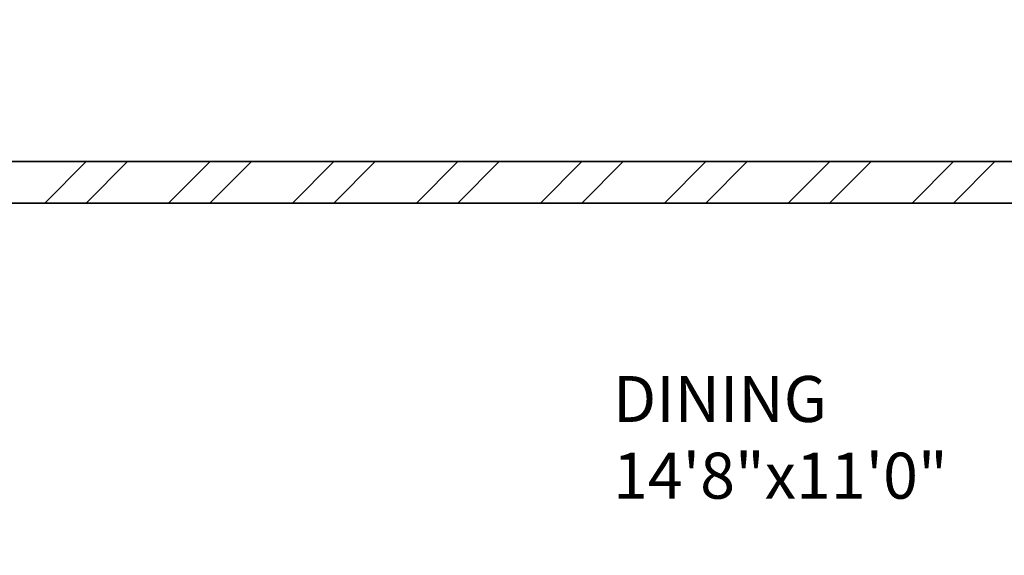
# Model space of a CAD drawing. Units: inches. Extents: x 1885 to 2748, y 783 to 2421.
# Tile 27 of 117: x 2338 to 2445, y 1292 to 1350. Entities that reach past the tile are written whole.
import ezdxf

# ---------------------------------------------------------------- set-up
doc = ezdxf.new("R2010")
doc.units = ezdxf.units.IN
doc.layers.add('A-AREA-IDEN', color=7, linetype='Continuous', lineweight=18)
doc.layers.add('A-WALL', color=7, linetype='Continuous', lineweight=35)
doc.layers.add('A-WALL-PATT', color=85, linetype='Continuous', lineweight=13, true_color=0x58ba48)
doc.styles.get("Standard").update_dxf_attribs({"font": 'arial.ttf'})

msp = doc.modelspace()

# ---------------------------------------------------------------- hatches: boundary and pattern name
at = {"layer": 'A-WALL-PATT'}
h = msp.add_hatch(dxfattribs=at)
h.set_pattern_fill('ANSI32', color=256)
h.paths.add_polyline_path([(2007.77, 2318.01), (1980.77, 2318.01), (1980.77, 2281.22), (1985.27, 2281.22), (1985.27, 2313.51), (2007.77, 2313.51), (2007.77, 2315.76)])
h.paths.add_polyline_path([(2094.32, 2318.01), (2067.77, 2318.01), (2067.77, 2313.51), (2094.32, 2313.51), (2094.32, 2315.76)])
h.paths.add_polyline_path([(2131.37, 2315.76), (2131.37, 2318.01), (2131.19, 2318.01), (2112.61, 2318.01), (2112.61, 2313.51), (2117.27, 2313.51), (2117.27, 2255.2), (2121.77, 2255.2), (2121.77, 2313.51), (2131.37, 2313.51)])
h.paths.add_polyline_path([(2190.51, 2318.01), (2155.37, 2318.01), (2155.37, 2313.51), (2169.77, 2313.51), (2169.77, 2229.51), (2121.77, 2229.51), (2121.77, 2233.45), (2119.52, 2233.45), (2117.27, 2233.45), (2117.27, 2201.1), (2121.77, 2201.1), (2121.77, 2225.01), (2169.77, 2225.01), (2169.77, 2165.01), (2306.27, 2165.01), (2306.27, 2066.01), (2310.77, 2066.01), (2344.27, 2066.01), (2486.27, 2066.01), (2486.27, 1886.01), (2483.02, 1886.01), (2483.02, 1881.51), (2486.27, 1881.51), (2486.27, 1880.68), (2490.77, 1880.68), (2490.77, 2070.51), (2344.27, 2070.51), (2310.77, 2070.51), (2310.77, 2165.01), (2310.77, 2173.64), (2308.52, 2173.64), (2306.27, 2173.64), (2306.27, 2169.51), (2174.27, 2169.51), (2174.27, 2313.51), (2190.51, 2313.51), (2190.51, 2315.76)])
h.paths.add_polyline_path([(1985.27, 2221.22), (1980.77, 2221.22), (1980.77, 2165.01), (1992.77, 2165.01), (1992.77, 2141.93), (1997.27, 2141.93), (1997.27, 2165.01), (2117.27, 2165.01), (2117.27, 2163.13), (2121.77, 2163.13), (2121.77, 2172.73), (2119.52, 2172.73), (2117.27, 2172.73), (2117.27, 2169.51), (1985.27, 2169.51)])
h.paths.add_polyline_path([(1997.27, 2105.93), (1992.77, 2105.93), (1992.77, 2070.51), (2016.77, 2070.51), (2016.77, 2059.12), (2019.02, 2059.12), (2021.27, 2059.12), (2021.27, 2070.51), (2117.27, 2070.51), (2117.27, 2022.51), (2114.42, 2022.51), (2114.42, 2018.01), (2123.63, 2018.01), (2123.63, 2020.26), (2123.63, 2022.51), (2121.77, 2022.51), (2121.77, 2142.59), (2119.52, 2142.59), (2117.27, 2142.59), (2117.27, 2075.01), (1997.27, 2075.01)])
h.paths.add_polyline_path([(2092.03, 2020.26), (2092.03, 2022.51), (2021.27, 2022.51), (2021.27, 2035.12), (2016.77, 2035.12), (2016.77, 2018.01), (2016.77, 1978.78), (2021.27, 1978.78), (2021.27, 2018.01), (2092.03, 2018.01)])
h.paths.add_polyline_path([(2260.94, 2022.51), (2153.1, 2022.51), (2153.1, 2020.26), (2153.1, 2018.01), (2155.27, 2018.01), (2155.27, 1886.01), (2107.63, 1886.01), (2107.63, 1881.51), (2182.91, 1881.51), (2182.91, 1883.76), (2182.91, 1886.01), (2159.77, 1886.01), (2159.77, 2018.01), (2260.94, 2018.01), (2260.94, 2020.26)])
h.paths.add_polyline_path([(2047.63, 1883.76), (2047.63, 1886.01), (2021.27, 1886.01), (2021.27, 1918.78), (2019.02, 1918.78), (2016.77, 1918.78), (2016.77, 1881.51), (2047.63, 1881.51)])
h.paths.add_polyline_path([(2306.36, 1883.76), (2306.36, 1886.01), (2296.27, 1886.01), (2296.27, 1982.01), (2316.54, 1982.01), (2316.54, 1984.26), (2316.54, 1986.51), (2296.27, 1986.51), (2296.27, 2022.51), (2289.28, 2022.51), (2289.28, 2018.01), (2291.77, 2018.01), (2291.77, 1886.01), (2242.91, 1886.01), (2242.91, 1881.51), (2306.36, 1881.51)], flags=17)
h.paths.add_polyline_path([(1985.27, 1843.01), (2021.6, 1843.01), (2021.53, 1845.44), (2021.48, 1847.51), (1980.77, 1847.51), (1980.77, 1809.45), (1985.27, 1809.45)])
h.paths.add_polyline_path([(2131.48, 1845.26), (2131.48, 1847.51), (2081.53, 1847.51), (2081.53, 1843.01), (2117.27, 1843.01), (2117.27, 1784.15), (2119.52, 1784.15), (2121.77, 1784.15), (2121.77, 1843.01), (2131.48, 1843.01)])
h.paths.add_polyline_path([(2203.89, 1847.51), (2155.48, 1847.51), (2155.48, 1843.01), (2169.77, 1843.01), (2169.77, 1759.01), (2121.77, 1759.01), (2121.77, 1761.46), (2117.27, 1761.46), (2117.27, 1730.43), (2121.77, 1730.43), (2121.77, 1754.51), (2177.42, 1754.51), (2177.42, 1756.76), (2177.42, 1759.01), (2174.27, 1759.01), (2174.27, 1843.01), (2203.89, 1843.01)])
h.paths.add_polyline_path([(2335.55, 1845.26), (2335.55, 1847.51), (2239.89, 1847.51), (2239.89, 1843.01), (2306.27, 1843.01), (2306.27, 1759.01), (2199.49, 1759.01), (2199.49, 1754.51), (2310.77, 1754.51), (2310.77, 1843.01), (2335.55, 1843.01)])
h.paths.add_polyline_path([(2348.77, 2022.51), (2344.27, 2022.51), (2344.27, 1986.51), (2341.68, 1986.51), (2341.68, 1982.01), (2344.27, 1982.01), (2344.27, 1886.01), (2330.36, 1886.01), (2330.36, 1881.51), (2361.63, 1881.51), (2361.63, 1883.76), (2361.63, 1886.01), (2348.77, 1886.01)], flags=17)
h.paths.add_polyline_path([(2283.25, 2315.76), (2283.25, 2318.01), (2238.51, 2318.01), (2238.51, 2313.51), (2283.25, 2313.51)], flags=17)
h.paths.add_polyline_path([(2363.27, 2348.01), (2388.68, 2348.01), (2388.68, 2350.26), (2388.68, 2352.51), (2358.77, 2352.51), (2358.77, 2348.01), (2358.77, 2318.01), (2344.48, 2318.01), (2344.48, 2313.51), (2358.77, 2313.51), (2358.77, 2229.51), (2310.77, 2229.51), (2310.77, 2231.95), (2306.27, 2231.95), (2306.27, 2205.61), (2310.77, 2205.61), (2310.77, 2225.01), (2358.77, 2225.01), (2358.77, 2211.51), (2452.33, 2211.51), (2452.33, 2213.76), (2452.33, 2216.01), (2363.27, 2216.01), (2363.27, 2318.01)])
h.paths.add_polyline_path([(2310.77, 2313.51), (2320.48, 2313.51), (2320.48, 2315.76), (2320.48, 2318.01), (2302.73, 2318.01), (2302.73, 2313.51), (2306.27, 2313.51), (2306.27, 2251.08), (2310.77, 2251.08)], flags=17)
h.paths.add_polyline_path([(2490.77, 2352.51), (2486.27, 2352.51), (2448.68, 2352.51), (2448.68, 2348.01), (2486.27, 2348.01), (2486.27, 2318.01), (2486.27, 2216.01), (2481.78, 2216.01), (2481.78, 2211.51), (2486.27, 2211.51), (2486.27, 2165.01), (2493.29, 2165.01), (2493.29, 2167.26), (2493.29, 2169.51), (2490.77, 2169.51), (2490.77, 2313.51), (2494.43, 2313.51), (2494.43, 2318.01), (2490.77, 2318.01)])
h.paths.add_polyline_path([(2534.65, 2318.01), (2515.69, 2318.01), (2515.69, 2313.51), (2534.65, 2313.51), (2534.65, 2315.76)])
h.paths.add_polyline_path([(2618.27, 2318.01), (2594.65, 2318.01), (2594.65, 2313.51), (2613.77, 2313.51), (2613.77, 2281.71), (2618.27, 2281.71)])
h.paths.add_polyline_path([(2618.27, 2221.71), (2613.77, 2221.71), (2613.77, 2169.51), (2554.02, 2169.51), (2554.02, 2165.01), (2613.77, 2165.01), (2613.77, 2152.88), (2618.27, 2152.88)])
h.paths.add_polyline_path([(2618.27, 2128.88), (2616.02, 2128.88), (2613.77, 2128.88), (2613.77, 2117.01), (2529.77, 2117.01), (2529.77, 2165.01), (2532.85, 2165.01), (2532.85, 2169.51), (2522.87, 2169.51), (2522.87, 2165.01), (2525.27, 2165.01), (2525.27, 2117.01), (2525.27, 2112.51), (2525.27, 2108.58), (2529.77, 2108.58), (2529.77, 2112.51), (2613.77, 2112.51), (2613.77, 2080.19), (2618.27, 2080.19)])
h.paths.add_polyline_path([(2618.27, 2044.19), (2616.02, 2044.19), (2613.77, 2044.19), (2613.77, 2015.51), (2529.77, 2015.51), (2529.77, 2088.58), (2527.52, 2088.58), (2525.27, 2088.58), (2525.27, 2011.01), (2613.77, 2011.01), (2613.77, 1956.75), (2618.27, 1956.75)])
h.paths.add_polyline_path([(2618.27, 1881.51), (2618.27, 1896.75), (2613.77, 1896.75), (2613.77, 1881.51), (2613.77, 1847.51), (2592.71, 1847.51), (2592.71, 1843.01), (2613.77, 1843.01), (2613.77, 1765.01), (2613.77, 1760.51), (2609.62, 1760.51), (2609.62, 1756.01), (2613.77, 1756.01), (2613.77, 1660.01), (2608.54, 1660.01), (2608.54, 1655.51), (2613.77, 1655.51), (2613.77, 1508.16), (2618.27, 1508.16)])
h.paths.add_polyline_path([(2565.77, 1843.01), (2569, 1843.01), (2569, 1847.51), (2490.77, 1847.51), (2490.77, 1849.7), (2488.52, 1849.7), (2486.27, 1849.7), (2486.27, 1847.51), (2477.27, 1847.51), (2477.27, 1838.51), (2477.27, 1821.49), (2486.27, 1821.49), (2486.27, 1838.51), (2561.27, 1838.51), (2561.27, 1765.01), (2486.27, 1765.01), (2486.27, 1786.16), (2477.27, 1786.16), (2477.27, 1765.01), (2477.27, 1756.01), (2486.27, 1756.01), (2565.77, 1756.01), (2585.62, 1756.01), (2585.62, 1758.26), (2585.62, 1760.51), (2565.77, 1760.51), (2565.77, 1765.01)])
h.paths.add_polyline_path([(2486.27, 1651.01), (2561.27, 1651.01), (2561.27, 1567.01), (2486.27, 1567.01), (2486.27, 1591.32), (2477.27, 1591.32), (2477.27, 1567.01), (2477.27, 1558.01), (2477.27, 1555.44), (2481.77, 1555.44), (2481.77, 1558.01), (2568.65, 1558.01), (2568.65, 1560.26), (2568.65, 1562.51), (2565.77, 1562.51), (2565.77, 1655.51), (2584.54, 1655.51), (2584.54, 1657.76), (2584.54, 1660.01), (2565.77, 1660.01), (2486.27, 1660.01), (2477.27, 1660.01), (2477.27, 1651.01), (2477.27, 1632.99), (2486.27, 1632.99)])
h.paths.add_polyline_path([(2449.97, 1883.76), (2449.97, 1886.01), (2421.63, 1886.01), (2421.63, 1881.51), (2449.97, 1881.51)], flags=17)
h.paths.add_polyline_path([(2447.27, 1847.51), (2395.55, 1847.51), (2395.55, 1843.01), (2442.77, 1843.01), (2442.77, 1809.27), (2447.27, 1809.27)])
h.paths.add_polyline_path([(1985.27, 1749.45), (1980.77, 1749.45), (1980.77, 1694.5), (1985.27, 1694.5), (1985.27, 1694.51), (1986.9, 1694.51), (1986.9, 1697.78), (1986.9, 1699.01), (1985.27, 1699.01)])
h.paths.add_polyline_path([(2152.77, 1699.01), (2121.77, 1699.01), (2121.77, 1703.67), (2119.52, 1703.67), (2117.27, 1703.67), (2117.27, 1699.01), (2009.22, 1699.01), (2009.22, 1694.51), (2148.27, 1694.51), (2148.27, 1692.63), (2152.77, 1692.63)])
h.paths.add_polyline_path([(2016.27, 1694.51), (2011.77, 1694.51), (2011.77, 1558.01), (2040.81, 1558.01), (2040.81, 1560.26), (2040.81, 1562.51), (2016.27, 1562.51)])
h.paths.add_polyline_path([(2152.77, 1663.02), (2150.52, 1663.02), (2148.27, 1663.02), (2148.27, 1562.51), (2100.81, 1562.51), (2100.81, 1558.01), (2165.12, 1558.01), (2165.12, 1560.26), (2165.12, 1562.51), (2152.77, 1562.51), (2152.77, 1610.51), (2224.77, 1610.51), (2224.77, 1607.99), (2229.27, 1607.99), (2229.27, 1615.01), (2152.77, 1615.01)])
h.paths.add_polyline_path([(2238.61, 1560.26), (2238.61, 1562.51), (2229.27, 1562.51), (2229.27, 1588.76), (2227.02, 1588.76), (2224.77, 1588.77), (2224.77, 1562.51), (2189.12, 1562.51), (2189.12, 1558.01), (2238.61, 1558.01)])
h.paths.add_polyline_path([(2336.02, 1560.26), (2336.02, 1562.51), (2310.77, 1562.51), (2310.77, 1656.35), (2308.52, 1656.35), (2306.27, 1656.35), (2306.27, 1562.51), (2286.61, 1562.51), (2286.61, 1558.01), (2336.02, 1558.01)])
h.paths.add_polyline_path([(2447.27, 1690.97), (2445.02, 1690.97), (2442.77, 1690.97), (2442.77, 1687.01), (2306.27, 1687.01), (2306.27, 1680.75), (2310.77, 1680.75), (2310.77, 1682.51), (2442.77, 1682.51), (2442.77, 1562.51), (2396.02, 1562.51), (2396.02, 1558.01), (2447.27, 1558.01)])
h.paths.add_polyline_path([(2447.27, 1749.27), (2445.02, 1749.27), (2442.77, 1749.27), (2442.77, 1717.23), (2447.27, 1717.23)])
h.paths.add_polyline_path([(2044.67, 1521.76), (2044.67, 1524.01), (2007.27, 1524.01), (2007.27, 1503.49), (2009.52, 1503.49), (2011.77, 1503.49), (2011.77, 1519.51), (2044.67, 1519.51)])
h.paths.add_polyline_path([(2177.97, 1521.76), (2177.97, 1524.01), (2104.67, 1524.01), (2104.67, 1519.51), (2145.77, 1519.51), (2145.77, 1387.51), (2143.37, 1387.51), (2143.37, 1383.01), (2251.59, 1383.01), (2251.59, 1385.26), (2251.59, 1387.51), (2150.27, 1387.51), (2150.27, 1519.51), (2177.97, 1519.51)])
h.paths.add_polyline_path([(2298.7, 1524.01), (2237.97, 1524.01), (2237.97, 1519.51), (2282.27, 1519.51), (2282.27, 1387.51), (2279.68, 1387.51), (2279.68, 1383.01), (2286.77, 1383.01), (2286.77, 1419.01), (2312.45, 1419.01), (2312.45, 1421.26), (2312.45, 1423.51), (2286.77, 1423.51), (2286.77, 1519.51), (2298.7, 1519.51), (2298.7, 1521.72)], flags=17)
h.paths.add_polyline_path([(2361.9, 1521.76), (2361.9, 1524.01), (2322.7, 1524.01), (2322.7, 1519.51), (2334.77, 1519.51), (2334.77, 1423.51), (2331.93, 1423.51), (2331.93, 1419.01), (2334.77, 1419.01), (2334.77, 1387.51), (2334.77, 1383.23), (2339.27, 1383.23), (2339.27, 1387.51), (2339.27, 1519.51), (2361.9, 1519.51)], flags=17)
h.paths.add_polyline_path([(2447.27, 1521.76), (2447.27, 1524.01), (2421.9, 1524.01), (2421.9, 1519.51), (2447.27, 1519.51)], flags=17)
h.paths.add_polyline_path([(2481.77, 1529.6), (2479.52, 1529.6), (2477.27, 1529.6), (2477.27, 1524.01), (2474.49, 1524.01), (2474.49, 1519.51), (2477.27, 1519.51), (2477.27, 1334.51), (2296.77, 1334.51), (2296.77, 1240.51), (2160.27, 1240.51), (2160.27, 1180.51), (2112.27, 1180.51), (2112.27, 1207.69), (2110.02, 1207.69), (2107.77, 1207.69), (2107.77, 1171.61), (2112.27, 1171.61), (2112.27, 1176.01), (2160.27, 1176.01), (2160.27, 1092.01), (2144.22, 1092.01), (2144.22, 1087.51), (2189.5, 1087.51), (2189.5, 1089.76), (2189.5, 1092.01), (2164.77, 1092.01), (2164.77, 1236.01), (2296.77, 1236.01), (2296.77, 1231.91), (2301.27, 1231.91), (2301.27, 1330.01), (2481.77, 1330.01), (2481.77, 1387.51)])
h.paths.add_polyline_path([(2618.27, 1448.16), (2613.77, 1448.16), (2613.77, 1382.51), (2529.77, 1382.51), (2525.27, 1382.51), (2525.27, 1307.06), (2529.77, 1307.06), (2529.77, 1378.01), (2613.77, 1378.01), (2613.77, 1354.99), (2618.27, 1354.99)])
h.paths.add_polyline_path([(2618.27, 1318.99), (2613.77, 1318.99), (2613.77, 1281.01), (2529.77, 1281.01), (2529.77, 1283.79), (2527.52, 1283.79), (2525.27, 1283.79), (2525.27, 1228.51), (2516.79, 1228.51), (2516.79, 1224.01), (2533.48, 1224.01), (2533.48, 1226.26), (2533.48, 1228.51), (2529.77, 1228.51), (2529.77, 1276.51), (2613.77, 1276.51), (2613.77, 1266.02), (2618.27, 1266.02)])
h.paths.add_polyline_path([(2618.27, 1134.96), (2613.77, 1134.96), (2613.77, 1092.01), (2594.54, 1092.01), (2594.54, 1087.51), (2618.27, 1087.51)])
h.paths.add_polyline_path([(2534.54, 1092.01), (2509.77, 1092.01), (2509.77, 1087.51), (2534.54, 1087.51), (2534.54, 1089.76)])
h.paths.add_polyline_path([(2481.27, 1224.01), (2484.12, 1224.01), (2484.12, 1226.26), (2484.12, 1228.51), (2476.77, 1228.51), (2476.77, 1198.51), (2471.61, 1198.51), (2471.61, 1194.01), (2476.77, 1194.01), (2476.77, 1062.01), (2436.89, 1062.01), (2436.89, 1057.51), (2476.77, 1057.51), (2481.27, 1057.51), (2481.27, 1062.01), (2481.27, 1087.51), (2485.35, 1087.51), (2485.35, 1089.76), (2485.35, 1092.01), (2481.27, 1092.01), (2481.27, 1117.51)])
h.paths.add_polyline_path([(2439.9, 1198.51), (2349.27, 1198.51), (2349.27, 1194.01), (2349.27, 1180.51), (2301.27, 1180.51), (2301.27, 1201.9), (2299.02, 1201.9), (2296.77, 1201.9), (2296.77, 1172.34), (2299.02, 1172.34), (2301.27, 1172.34), (2301.27, 1176.01), (2349.27, 1176.01), (2349.27, 1092.01), (2334.45, 1092.01), (2334.45, 1087.51), (2349.27, 1087.51), (2349.27, 1057.51), (2353.77, 1057.51), (2376.89, 1057.51), (2376.89, 1059.76), (2376.89, 1062.01), (2353.77, 1062.01), (2353.77, 1087.51), (2353.77, 1180.51), (2353.77, 1194.01), (2439.9, 1194.01), (2439.9, 1196.26)])
h.paths.add_polyline_path([(2270.6, 1089.76), (2270.6, 1092.01), (2249.5, 1092.01), (2249.5, 1087.51), (2270.6, 1087.51)], flags=17)
h.paths.add_polyline_path([(2310.45, 1092.01), (2301.27, 1092.01), (2301.27, 1153.29), (2296.77, 1153.29), (2296.77, 1092.01), (2293.79, 1092.01), (2293.79, 1087.51), (2310.45, 1087.51), (2310.45, 1089.76)], flags=17)
h.paths.add_polyline_path([(2112.27, 1150.33), (2110.02, 1150.33), (2107.77, 1150.33), (2107.77, 1092.01), (2104.47, 1092.01), (2104.47, 1087.51), (2120.22, 1087.51), (2120.22, 1089.76), (2120.22, 1092.01), (2112.27, 1092.01)])
h.paths.add_polyline_path([(2082.17, 1092.01), (2058.14, 1092.01), (2058.14, 1087.51), (2082.17, 1087.51), (2082.17, 1089.76)])
h.paths.add_polyline_path([(1975.77, 1145.64), (1971.27, 1145.64), (1971.27, 1087.51), (1980.77, 1087.51), (1998.14, 1087.51), (1998.14, 1089.76), (1998.14, 1092.01), (1985.27, 1092.01), (1975.77, 1092.01)])
h.paths.add_polyline_path([(2112.27, 1244.38), (2110.02, 1244.38), (2107.77, 1244.38), (2107.77, 1240.51), (1992.27, 1240.51), (1992.27, 1271.01), (1987.77, 1271.01), (1987.77, 1240.51), (1980.77, 1240.51), (1975.77, 1240.51), (1971.27, 1240.51), (1971.27, 1205.64), (1975.77, 1205.64), (1975.77, 1236.01), (2107.77, 1236.01), (2107.77, 1233.44), (2112.27, 1233.44), (2112.27, 1236.01)])
h.paths.add_polyline_path([(2112.27, 1383.01), (2114.78, 1383.01), (2114.78, 1385.26), (2114.78, 1387.51), (2102.48, 1387.51), (2102.48, 1383.01), (2107.77, 1383.01), (2107.77, 1335.01), (2011.77, 1335.01), (2011.77, 1349.94), (2007.27, 1349.94), (2007.27, 1335.01), (1987.77, 1335.01), (1987.77, 1330.51), (1987.77, 1307.01), (1992.27, 1307.01), (1992.27, 1330.51), (2007.27, 1330.51), (2107.77, 1330.51), (2107.77, 1264.71), (2112.27, 1264.71)])
h.paths.add_polyline_path([(2077.86, 1387.51), (2011.77, 1387.51), (2011.77, 1390.04), (2009.52, 1390.04), (2007.27, 1390.04), (2007.27, 1373.94), (2011.77, 1373.94), (2011.77, 1383.01), (2077.86, 1383.01)])
h.paths.add_polyline_path([(2011.77, 1443.49), (2007.27, 1443.49), (2007.27, 1410.25), (2011.77, 1410.25)])

# ---------------------------------------------------------------- linework, layer by layer
at = {"layer": 'A-WALL'}
for p, q in [((2477.27, 1334.51), (2296.77, 1334.51)), ((2301.27, 1330.01), (2481.77, 1330.01))]:
    msp.add_line(p, q, dxfattribs=at)

# ---------------------------------------------------------------- texts
at = {"layer": 'A-AREA-IDEN', "insert": (2402.06, 1311.21), "char_height": 5, "attachment_point": 1}
msp.add_mtext_dynamic_manual_height_columns('DINING\\P14\'8"x11\'0"', width=142.0662, gutter_width=12.5, heights=[0], dxfattribs=at)

doc.saveas('drawing.dxf')
